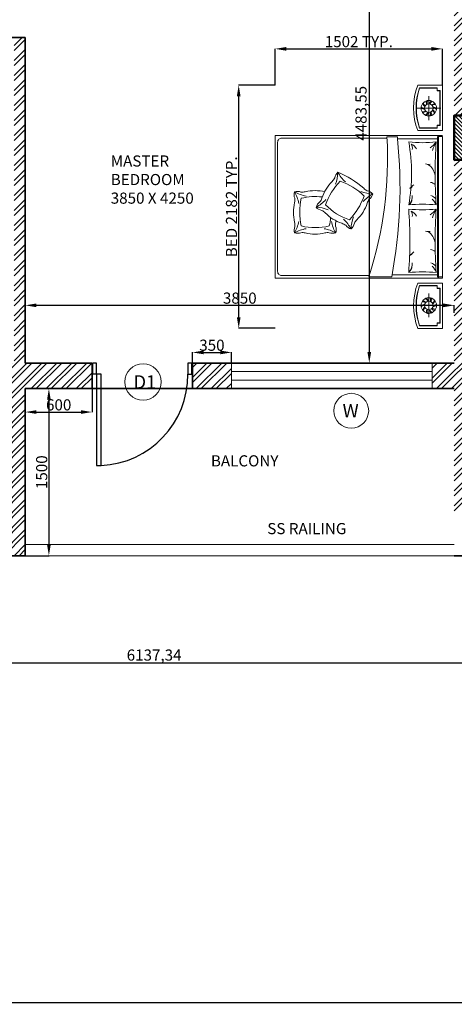
# Model space of a CAD drawing. Units: millimetres. Extents: x -3326 to 29338, y -16792 to 6002.
# Tile 5 of 21: x 7252 to 11152, y -16792 to -7951. Entities that reach past the tile are written whole.
import ezdxf

# ---------------------------------------------------------------- set-up
doc = ezdxf.new("R2010")
doc.units = ezdxf.units.MM
doc.header["$PDMODE"] = 35
doc.header["$PDSIZE"] = 5
for name, color, linetype, lineweight in [('A-ANNO-DIMS', 2, 'Continuous', 13), ('A-ANNO-SYMB', 7, 'Continuous', 18), ('A-AREA-IDEN', 7, 'Continuous', 18), ('A-COLS', 1, 'Continuous', 50), ('A-COLS-PATT', 251, 'Continuous', 13), ('A-DOOR', 3, 'Continuous', 25), ('A-FLOR-RAIL', 8, 'Continuous', 20), ('A-GLAZ', 4, 'Continuous', 18), ('A-WALL', 7, 'Continuous', 35), ('A-WALL-PATT', 252, 'Continuous', 13), ('furn', 28, 'Continuous', 18), ('txt', 7, 'Continuous', 18)]:
    doc.layers.add(name, color=color, linetype=linetype, lineweight=lineweight)
doc.styles.get("Standard").update_dxf_attribs({"font": 'arial.ttf'})
doc.dimstyles.new('ISO-25', dxfattribs={"dimtxt": 100, "dimasz": 100, "dimexe": 1.25, "dimexo": 0.625, "dimtad": 1, "dimtxsty": 'Standard', "dimcen": 2.5, "dimadec": 0, "dimazin": 0, "dimtfac": 1, "dimtmove": 0, "dimatfit": 3, "dimfxl": 1, "dimarcsym": 0})
pattern_1 = [(45, (-10476.65, 1e-12), (-67.35192, 67.35192), []), (45, (-10431.74, 1e-12), (-67.35192, 67.35192), [])]

# ---------------------------------------------------------------- blocks, each defined once
blk = doc.blocks.new('A$C0CE462CD')
for p, q in [((860, 100), (860, 0)), ((860, 0), (893.9, 0))]:
    blk.add_line(p, q)
for points in [[(860, 100), (860, 920), (818.4, 920), (818.4, 100)], [(0, 10), (6.1, 10), (6.1, 90), (0, 90)], [(893.9, 10), (900, 10), (900, 90), (893.9, 90)]]:
    blk.add_lwpolyline(points, close=True)
for points in [[(6.1, 0), (40, 0), (40, 100), (6.1, 100)], [(6.1, 100), (6.1, 0)], [(860, 100), (893.9, 100), (893.9, 0)]]:
    blk.add_lwpolyline(points)
blk.add_arc((859.1, 101.9), 819.1, 92.8508, 180.13091)
blk = doc.blocks.new('*D55')
at = {"layer": 'A-ANNO-DIMS', "color": 0, "lineweight": -2, "transparency": 16777216}
for p, q in [((7302.9, -11264), (7515.4, -11264)), ((7514.2, -11364), (7514.2, -12664)), ((7302.9, -12764), (7515.4, -12764))]:
    blk.add_line(p, q, dxfattribs=at)
at = {"layer": 'A-ANNO-DIMS', "color": 0, "transparency": 16777216}
for points in [[(7497.5, -11364), (7530.8, -11364), (7514.2, -11264)], [(7497.5, -12664), (7530.8, -12664), (7514.2, -12764)]]:
    blk.add_solid(points, dxfattribs=at)
at = {"layer": 'Defpoints', "color": 0, "transparency": 16777216}
for p in [(7302.3, -11264), (7302.3, -12764), (7514.2, -12764)]:
    blk.add_point(p, dxfattribs=at)
at = {"layer": 'A-ANNO-DIMS', "color": 0, "transparency": 16777216, "insert": (7462.5, -12014), "char_height": 100, "attachment_point": 5, "rotation": 90}
blk.add_mtext('1500', dxfattribs=at)
blk = doc.blocks.new('*D56')
at = {"layer": 'A-ANNO-DIMS', "color": 0, "lineweight": -2, "transparency": 16777216}
for p, q in [((8802.3, -11033.3), (8802.3, -10937.6)), ((8902.3, -10938.8), (9052.3, -10938.8)), ((9152.3, -11033.3), (9152.3, -10937.6))]:
    blk.add_line(p, q, dxfattribs=at)
at = {"layer": 'A-ANNO-DIMS', "color": 0, "transparency": 16777216}
for points in [[(8902.3, -10922.1), (8902.3, -10955.5), (8802.3, -10938.8)], [(9052.3, -10922.1), (9052.3, -10955.5), (9152.3, -10938.8)]]:
    blk.add_solid(points, dxfattribs=at)
at = {"layer": 'Defpoints', "color": 0, "transparency": 16777216}
for p in [(9152.3, -10938.8), (8802.3, -11034), (9152.3, -11034)]:
    blk.add_point(p, dxfattribs=at)
at = {"layer": 'A-ANNO-DIMS', "color": 0, "transparency": 16777216, "insert": (8977.3, -10887.1), "char_height": 100, "attachment_point": 5}
blk.add_mtext('350', dxfattribs=at)
blk = doc.blocks.new('*D57')
at = {"layer": 'A-ANNO-DIMS', "color": 0, "lineweight": -2, "transparency": 16777216}
for p, q in [((7302.3, -11264.6), (7302.3, -11475.4)), ((7902.3, -11264.6), (7902.3, -11475.4)), ((7402.3, -11474.2), (7802.3, -11474.2))]:
    blk.add_line(p, q, dxfattribs=at)
at = {"layer": 'A-ANNO-DIMS', "color": 0, "transparency": 16777216}
for points in [[(7402.3, -11457.5), (7402.3, -11490.8), (7302.3, -11474.2)], [(7802.3, -11457.5), (7802.3, -11490.8), (7902.3, -11474.2)]]:
    blk.add_solid(points, dxfattribs=at)
at = {"layer": 'Defpoints', "color": 0, "transparency": 16777216}
for p in [(7302.3, -11264), (7902.3, -11264), (7902.3, -11474.2)]:
    blk.add_point(p, dxfattribs=at)
at = {"layer": 'A-ANNO-DIMS', "color": 0, "transparency": 16777216, "insert": (7602.3, -11422.5), "char_height": 100, "attachment_point": 5}
blk.add_mtext('600', dxfattribs=at)
blk = doc.blocks.new('*D58')
at = {"layer": 'A-ANNO-DIMS', "color": 0, "lineweight": -2, "transparency": 16777216}
for p, q in [((7302.3, -10583), (7302.3, -10514.7)), ((7402.3, -10515.9), (11052.3, -10515.9)), ((11152.3, -10583), (11152.3, -10514.7))]:
    blk.add_line(p, q, dxfattribs=at)
at = {"layer": 'A-ANNO-DIMS', "color": 0, "transparency": 16777216}
for points in [[(7402.3, -10499.2), (7402.3, -10532.6), (7302.3, -10515.9)], [(11052.3, -10499.2), (11052.3, -10532.6), (11152.3, -10515.9)]]:
    blk.add_solid(points, dxfattribs=at)
at = {"layer": 'Defpoints', "color": 0, "transparency": 16777216}
for p in [(11152.3, -10515.9), (7302.3, -10583.6), (11152.3, -10583.6)]:
    blk.add_point(p, dxfattribs=at)
at = {"layer": 'A-ANNO-DIMS', "color": 0, "transparency": 16777216, "insert": (9227.3, -10464.2), "char_height": 100, "attachment_point": 5}
blk.add_mtext('3850', dxfattribs=at)
blk = doc.blocks.new('*D59')
at = {"layer": 'A-ANNO-DIMS', "color": 0, "lineweight": -2, "transparency": 16777216}
for p, q in [((10416, -6550.4), (10388, -6550.4)), ((10389.2, -6650.4), (10389.2, -10934)), ((10416, -11034), (10388, -11034))]:
    blk.add_line(p, q, dxfattribs=at)
at = {"layer": 'A-ANNO-DIMS', "color": 0, "transparency": 16777216}
for points in [[(10372.6, -6650.4), (10405.9, -6650.4), (10389.2, -6550.4)], [(10372.6, -10934), (10405.9, -10934), (10389.2, -11034)]]:
    blk.add_solid(points, dxfattribs=at)
at = {"layer": 'Defpoints', "color": 0, "transparency": 16777216}
for p in [(10416.6, -6550.4), (10389.2, -11034), (10416.6, -11034)]:
    blk.add_point(p, dxfattribs=at)
at = {"layer": 'A-ANNO-DIMS', "color": 0, "transparency": 16777216, "insert": (10328.5, -8792.2), "char_height": 100, "attachment_point": 5, "rotation": 90}
blk.add_mtext('4483,55', dxfattribs=at)
blk = doc.blocks.new('*D160')
at = {"layer": 'A-ANNO-DIMS', "color": 0, "lineweight": -2, "transparency": 16777216}
for p, q in [((5390, -13729), (5390, -13728.4)), ((11427.3, -13729.7), (5490, -13729.7)), ((11527.3, -13729), (11527.3, -13728.4))]:
    blk.add_line(p, q, dxfattribs=at)
at = {"layer": 'A-ANNO-DIMS', "color": 0, "transparency": 16777216}
for points in [[(5490, -13713), (5490, -13746.3), (5390, -13729.7)], [(11427.3, -13713), (11427.3, -13746.3), (11527.3, -13729.7)]]:
    blk.add_solid(points, dxfattribs=at)
at = {"layer": 'Defpoints', "color": 0, "transparency": 16777216}
for p in [(5390, -13729.7), (5390, -13729.7), (11527.3, -13729.7)]:
    blk.add_point(p, dxfattribs=at)
at = {"layer": 'A-ANNO-DIMS', "color": 0, "transparency": 16777216, "insert": (8458.6, -13668.9), "char_height": 100, "attachment_point": 5}
blk.add_mtext('6137,34', dxfattribs=at)
blk = doc.blocks.new('BED-WITH-NIGHTSTANDS')
for p, q in [((1378.9, 2083.2), (1378.9, 1869.8)), ((1272.3, 1976.5), (1485.6, 1976.5)), ((1466.8, 1702.3), (1097.4, 1702.3)), ((1455.8, 1708.6), (1455.8, 473.4)), ((1466.8, 480.5), (1049.3, 480.5)), ((1378.9, 98.8), (1378.9, 312.2)), ((1272.2, 205.5), (1485.6, 205.5))]:
    blk.add_line(p, q)
for points in [[(1279.5, 2182), (1501.4, 2182), (1501.4, 1775.2), (1279.5, 1775.2, -0.181818)], [(1097.4, 1719.6), (1097.4, 1702.3, -0.072944), (1045.8, 463.1), (840.6, 463.1, 0.092568), (1003.3, 1719.6)], [(1198.4, 1674.1, 0.058596), (1445.6, 1674.1, 0.036889), (1445.6, 1107.7, 0.052163), (1198.4, 1107.7, 0.093111)], [(1198.4, 1070.9, 0.058596), (1445.6, 1070.9, 0.036648), (1445.6, 500.8, 0.052163), (1198.4, 500.8, 0.036967)], [(1279.6, 0), (1501.5, 0), (1501.5, 406.8), (1279.6, 406.8, 0.181818)]]:
    blk.add_lwpolyline(points, format="xyb", close=True)
for points in [[(1454.8, 1797.4), (1295, 1797.4, -0.167087), (1295, 2159.8), (1454.8, 2159.8)], [(1454.8, 1799.6), (1296.6, 1799.6, -0.165559), (1296.6, 2157.6), (1454.8, 2157.6)], [(1003.9, 1708.6), (59.2, 1708.6, 0.414214), (22.2, 1671.6), (22.2, 510.4, 0.414214), (59.2, 473.4), (844.2, 473.4)], [(540, 1293.1, 0.091296), (562.8, 1401.4, 0.091296), (630.7, 1314.1, 0.091296)], [(583.2, 1320, 0.111006), (451.8, 1108.7, 0.119549), (665.6, 975.5, 0.107813), (797.5, 1186.1)], [(797.2, 1187.3, 0.121865), (583.2, 1319.9, 0.121865)], [(211.2, 1122.2, 0.091296), (173.3, 1226.2, 0.091296), (277.2, 1187.9, 0.091296)], [(233.7, 1167.8, 0.111006), (234, 919, 0.119549), (485.8, 919, 0.033212), (497.4, 995.5)], [(475.6, 1065.1, 0.091296), (367.2, 1087.5, 0.091296), (454.4, 1155.8)], [(768.3, 1228.3, 0.091296), (876.7, 1205.8, 0.091296), (789.5, 1137.6, 0.091296)], [(367.2, 1087.5, 0.159461), (418, 1058.9, -0.076283), (449.6, 1036.2, 0.115075), (598.7, 943.3, -0.076283), (633, 924.9, 0.159461), (681.1, 892)], [(703.9, 1000.2, 0.091296), (681.1, 892, 0.091296), (613.2, 979.3, 0.091296)], [(277.2, 894.6, 0.091296), (173.3, 856.3, 0.091296), (211.2, 960.3)], [(505.3, 960.3, 0.091296), (543.2, 856.3, 0.091296), (439.3, 894.6, 0.091296)], [(173.3, 856.3, 0.159461), (231.6, 858.9, -0.076283), (270.5, 856.3, 0.115075), (446, 856.3, -0.076283), (484.9, 858.9, 0.159461), (543.2, 856.3)], [(1454.9, 384.6), (1295.1, 384.6, 0.167087), (1295.1, 22.2), (1454.9, 22.2)], [(1454.9, 382.4), (1296.7, 382.4, 0.165559), (1296.7, 24.4), (1454.9, 24.4)]]:
    blk.add_lwpolyline(points, format="xyb")
for points in [[(1479.2, 2133.2), (1452.6, 2133.2), (1452.6, 2159.8)], [(1479.2, 2135.4), (1454.8, 2135.4), (1454.8, 2159.8)], [(1477, 2135.4), (1477, 1821.8)], [(1479.2, 2135.4), (1479.2, 1821.8)], [(1479.2, 1824), (1452.6, 1824), (1452.6, 1797.4)], [(1479.2, 1821.8), (1454.8, 1821.8), (1454.8, 1797.4)], [(1501.5, 1730.8), (0, 1730.8), (0, 451.2), (1501.5, 451.2)], [(1501.5, 463.1), (1466.8, 463.1), (1466.8, 1723.4), (1501.5, 1723.4), (1501.5, 451.2)], [(1479.3, 358), (1452.7, 358), (1452.7, 384.6)], [(1479.3, 360.2), (1454.9, 360.2), (1454.9, 384.6)], [(1477.1, 46.6), (1477.1, 360.2)], [(1479.3, 46.6), (1479.3, 360.2)], [(1479.3, 48.8), (1452.7, 48.8), (1452.7, 22.2)], [(1479.3, 46.6), (1454.9, 46.6), (1454.9, 22.2)]]:
    blk.add_lwpolyline(points)
for centre, radius in [((1378.9, 1976.5), 69.7), ((1378.9, 1976.5), 37.8), ((1378.9, 205.5), 69.7), ((1378.9, 205.5), 37.8)]:
    blk.add_circle(centre, radius)
for centre, radius, start, end in [((1400.9, 2024.2), 44.8, 154.17003, 200.48975), ((1396.5, 2024.6), 34.1, 142.30017, 202.53802), ((1424.8, 2002.2), 44.8, 118.17003, 164.48975), ((1421.4, 2005.1), 34.1, 106.30017, 166.53802), ((1340.3, 2012.2), 44.8, 226.17003, 272.48975), ((1338.5, 2008.1), 34.1, 214.30017, 274.53802), ((1327.7, 1978.3), 34.1, 250.30017, 310.53802), ((1326.7, 1982.7), 44.8, 262.17003, 308.48975), ((1368.7, 2028), 44.8, 190.17003, 236.48975), ((1364.8, 2025.8), 34.1, 178.30017, 238.53802), ((1431.1, 1970.3), 44.8, 82.17003, 128.48975), ((1430.1, 1974.7), 34.1, 70.30017, 130.53802), ((1393, 1927.2), 34.1, 358.30017, 58.53802), ((1389.2, 1925), 44.8, 10.17003, 56.48975), ((1417.5, 1940.8), 44.8, 46.17003, 92.48975), ((1419.3, 1944.9), 34.1, 34.30017, 94.53802), ((1336.4, 1947.9), 34.1, 286.30017, 346.53802), ((1333.1, 1950.8), 44.8, 298.17003, 344.48975), ((1361.4, 1928.3), 34.1, 322.30017, 22.53802), ((1356.9, 1928.8), 44.8, 334.17003, 20.48975), ((1478, 1708.6), 22.2, 90, 180), ((1175.6, 1619.4), 56.2, 346.48229, 38.55627), ((1192.7, 1576.7), 82.2, 24.2916, 70.9896), ((1214.5, 1859.4), 296.3, 306.49353, 321.27919), ((1652.3, 1542.6), 244.9, 147.53791, 167.5233), ((1375.3, 1532.7), 61.4, 245.89274, 286.11919), ((1299.1, 1354.7), 137.1, 6.68493, 58.3182), ((419.7, 1408.4), 128.4, 315.77185, 333.2208), ((626.3, 1332.5), 93.8, 132.65224, 168.89294), ((256.3, 651.7), 810, 48.38179, 67.76439), ((785.6, 1046.2), 386.5, 135.13065, 161.38844), ((884.1, 1348.9), 128.4, 225.58539, 243.03435), ((1208.9, 1279), 20.7, 263.75428, 347.21866), ((1026.5, 1507.4), 308.8, 306.20852, 315.08491), ((1377, 1216.1), 96.2, 51.81741, 79.89867), ((263.7, 1201.2), 93.8, 164.57915, 200.81985), ((198.5, 1135.9), 93.8, 69.36661, 105.60731), ((48.2, 1156.4), 128.4, 347.69876, 5.14771), ((242.7, 1351.6), 128.4, 265.03874, 282.4877), ((360.8, 659.2), 524.3, 83.19556, 104.02838), ((358.2, 849.8), 386.5, 76.87111, 103.12889), ((298.1, 1211.9), 128.4, 323.29829, 340.74724), ((807.5, 1142.5), 93.8, 42.46578, 78.70648), ((947.4, 1081.9), 128.4, 143.29829, 160.74724), ((789.7, 1230.6), 90.5, 307.29372, 344.09733), ((1127.7, 1179.9), 101.1, 314.40604, 6.83423), ((1163, 1161), 64, 303.63488, 0.84559), ((1363.4, 1094.5), 103.5, 40.53543, 70.35581), ((1276.2, 1030), 186.4, 24.64565, 44.15848), ((550.3, 1042.5), 386.5, 167.05756, 193.31535), ((468.2, 1051.5), 107.3, 128.77541, 160.35713), ((460, 1247.6), 386.5, 315.13065, 341.38844), ((1214.5, 1256.2), 296.3, 306.49353, 321.27919), ((1652.3, 939.4), 244.9, 147.53791, 167.5233), ((825.9, 885.4), 128.4, 135.77185, 153.2208), ((1175.6, 1016.2), 56.2, 346.48229, 38.55627), ((1192.7, 973.5), 82.2, 24.2916, 70.9896), ((278.1, 879.2), 107.3, 160.70232, 192.28404), ((48.9, 925.3), 128.4, 355.2252, 12.67415), ((669.5, 927.3), 128.4, 167.69876, 185.14771), ((461.1, 884), 86.6, 341.39955, 21.57741), ((167.4, 1041.2), 386.5, 347.05756, 348.7033), ((626.1, 958.8), 86.6, 309.47264, 349.6505), ((1375.3, 929.5), 61.4, 245.89274, 286.11919), ((1299.1, 751.6), 137.1, 6.68493, 58.3182), ((1377, 612.9), 96.2, 51.81741, 79.89867), ((1208.9, 675.8), 20.7, 263.75428, 347.21866), ((1026.5, 904.2), 308.8, 306.20852, 315.08491), ((1127.7, 576.7), 101.1, 314.40604, 6.83423), ((1163, 557.8), 64, 303.63488, 0.84559), ((1363.4, 491.3), 103.5, 40.53543, 70.35581), ((1276.2, 426.8), 186.4, 24.64565, 44.15848), ((1478, 473.4), 22.2, 180, 270), ((1336.4, 234.2), 34.1, 13.46198, 73.69983), ((1333, 231.2), 44.8, 15.51025, 61.82997), ((1361.4, 253.7), 34.1, 337.46198, 37.69983), ((1356.9, 253.2), 44.8, 339.51025, 25.82997), ((1340.3, 169.8), 44.8, 87.51025, 133.82997), ((1338.5, 173.9), 34.1, 85.46198, 145.69983), ((1327.7, 203.7), 34.1, 49.46198, 109.69983), ((1326.7, 199.3), 44.8, 51.51025, 97.82997), ((1368.6, 154), 44.8, 123.51025, 169.82997), ((1364.8, 156.2), 34.1, 121.46198, 181.69983), ((1430.1, 207.3), 34.1, 229.46198, 289.69983), ((1393, 254.8), 34.1, 301.46198, 1.69983), ((1389.2, 257.1), 44.8, 303.51025, 349.82997), ((1417.5, 241.2), 44.8, 267.51025, 313.82997), ((1419.3, 237.1), 34.1, 265.46198, 325.69983), ((1402.8, 152.7), 44.8, 159.51025, 205.82997), ((1398.4, 152.3), 34.1, 157.46198, 217.69983), ((1426.7, 174.7), 44.8, 195.51025, 241.82997), ((1423.3, 171.8), 34.1, 193.46198, 253.69983), ((1433, 206.6), 44.8, 231.51025, 277.82997)]:
    blk.add_arc(centre, radius, start, end)
blk = doc.blocks.new('TAG-D1')
blk.add_circle((163.3, 163.3), 163.3)
at = {"insert": (78, 223.5), "char_height": 120, "attachment_point": 1}
blk.add_mtext_dynamic_manual_height_columns('D1', width=137.943, gutter_width=12.5, heights=[0], dxfattribs=at)
blk = doc.blocks.new('TAG-W')
blk.add_circle((156.8, 156.8), 156.8)
at = {"insert": (79.7, 216.8), "char_height": 120, "attachment_point": 1}
blk.add_mtext_dynamic_manual_height_columns('W', width=376.575, gutter_width=12.5, heights=[0], dxfattribs=at)
blk = doc.blocks.new('GLAZ-1800x80')
for p, q in [((0, 80), (1800, 80)), ((0, 0), (1800, 0))]:
    blk.add_line(p, q)
blk = doc.blocks.new('*D213')
at = {"layer": 'A-ANNO-DIMS', "color": 0, "lineweight": -2, "transparency": 16777216}
for p, q in [((9544.2, -8540.5), (9216.3, -8540.5)), ((9217.5, -10622.5), (9217.5, -8640.5)), ((9544.2, -10722.5), (9216.3, -10722.5))]:
    blk.add_line(p, q, dxfattribs=at)
at = {"layer": 'A-ANNO-DIMS', "color": 0, "transparency": 16777216}
for points in [[(9200.9, -8640.5), (9234.2, -8640.5), (9217.5, -8540.5)], [(9200.9, -10622.5), (9234.2, -10622.5), (9217.5, -10722.5)]]:
    blk.add_solid(points, dxfattribs=at)
at = {"layer": 'Defpoints', "color": 0, "transparency": 16777216}
for p in [(9217.5, -8540.5), (9544.8, -8540.5), (9544.8, -10722.5)]:
    blk.add_point(p, dxfattribs=at)
at = {"layer": 'A-ANNO-DIMS', "color": 0, "transparency": 16777216, "insert": (9165.8, -9631.5), "char_height": 100, "attachment_point": 5, "rotation": 90}
blk.add_mtext('BED 2182 TYP.', dxfattribs=at)
blk = doc.blocks.new('*D214')
at = {"layer": 'A-ANNO-DIMS', "color": 0, "lineweight": -2, "transparency": 16777216}
for p, q in [((9544.8, -8539.9), (9544.8, -8212)), ((9644.8, -8213.2), (10946.3, -8213.2)), ((11046.3, -8539.9), (11046.3, -8212))]:
    blk.add_line(p, q, dxfattribs=at)
at = {"layer": 'A-ANNO-DIMS', "color": 0, "transparency": 16777216}
for points in [[(9644.8, -8196.5), (9644.8, -8229.9), (9544.8, -8213.2)], [(10946.3, -8196.5), (10946.3, -8229.9), (11046.3, -8213.2)]]:
    blk.add_solid(points, dxfattribs=at)
at = {"layer": 'Defpoints', "color": 0, "transparency": 16777216}
for p in [(11046.3, -8213.2), (9544.8, -8540.5), (11046.3, -8540.5)]:
    blk.add_point(p, dxfattribs=at)
at = {"layer": 'A-ANNO-DIMS', "color": 0, "transparency": 16777216, "insert": (10295.6, -8161.5), "char_height": 100, "attachment_point": 5}
blk.add_mtext('1502 TYP.', dxfattribs=at)
blk = doc.blocks.new('*D235')
at = {"layer": 'A-ANNO-DIMS', "color": 0, "lineweight": -2, "transparency": 16777216}
for p, q in [((-617.7, -12764.6), (-617.7, -16776.1)), ((29282.3, -12764.6), (29282.3, -16776.1)), ((-517.7, -16774.9), (29182.3, -16774.9))]:
    blk.add_line(p, q, dxfattribs=at)
at = {"layer": 'A-ANNO-DIMS', "color": 0, "transparency": 16777216}
for points in [[(-517.7, -16758.2), (-517.7, -16791.6), (-617.7, -16774.9)], [(29182.3, -16758.2), (29182.3, -16791.6), (29282.3, -16774.9)]]:
    blk.add_solid(points, dxfattribs=at)
at = {"layer": 'Defpoints', "color": 0, "transparency": 16777216}
for p in [(-617.7, -12764), (29282.3, -12764), (29282.3, -16774.9)]:
    blk.add_point(p, dxfattribs=at)
at = {"layer": 'A-ANNO-DIMS', "color": 0, "transparency": 16777216, "insert": (14332.3, -16723.2), "char_height": 100, "attachment_point": 5}
blk.add_mtext('29900', dxfattribs=at)

msp = doc.modelspace()

# ---------------------------------------------------------------- hatches: boundary and pattern name
at = {"layer": 'A-COLS-PATT'}
h = msp.add_hatch(dxfattribs=at)
h.set_pattern_fill('ANSI31', color=256, scale=8, angle=-90)
h.set_pattern_definition([(315, (18358.179, 32910.899), (17.960512, 17.960512), [])])
h.paths.add_polyline_path([(11151.174, -8810.401), (11151.174, -9210.401), (11751.174, -9210.401), (11751.174, -8810.401)])
at = {"layer": 'A-WALL-PATT'}
h = msp.add_hatch(dxfattribs=at)
h.set_pattern_fill('ANSI32', color=256, scale=10)
h.set_pattern_definition(pattern_1)
h.paths.add_polyline_path([(12212.301, -1983.952), (11640.861, -1983.952), (11640.861, -2213.952), (12212.301, -2213.952)])
h.paths.add_polyline_path([(14712.301, -1983.952), (14012.301, -1983.952), (14012.301, -2213.952), (14712.301, -2213.952)])
h.paths.add_polyline_path([(17012.301, -1983.952), (16512.301, -1983.952), (16512.301, -2213.952), (17012.301, -2213.952)])
h.paths.add_polyline_path([(11382.301, -2383.952), (11040.861, -2383.952), (7302.301, -2383.952), (7302.301, -1935.766), (7217.026, -1935.766), (7202.301, -1933.952), (7202.301, -2483.952), (7302.301, -2483.952), (11152.301, -2483.952), (11152.301, -2833.952), (11283.549, -2833.952), (11283.549, -2830.395), (11363.875, -2830.395), (11382.301, -2833.952)])
h.paths.add_polyline_path([(11382.301, -3733.952), (11363.875, -3733.952), (11363.875, -3734.058), (11283.549, -3734.058), (11152.301, -3733.952), (11152.301, -6450.401), (11382.301, -6450.401)])
h.paths.add_polyline_path([(13462.301, -6450.401), (12606.738, -6450.401), (11382.301, -6450.401), (11382.301, -6680.401), (12606.738, -6680.401), (13462.301, -6680.401)])
h.paths.add_polyline_path([(11382.301, -7050.401), (11152.301, -7050.401), (11152.301, -8810.401), (11382.301, -8810.401)])
h.paths.add_polyline_path([(13462.301, -8980.401), (11751.174, -8980.401), (11751.174, -9210.401), (13462.301, -9210.401)])
h.paths.add_polyline_path([(13962.301, -6850.401), (13732.301, -6850.401), (13732.301, -7350.401), (13962.301, -7350.401)])
h.paths.add_polyline_path([(13962.301, -8309.482), (13732.301, -8309.482), (13732.301, -8809.482), (13962.301, -8809.482)])
h.paths.add_polyline_path([(15712.301, -12533.952), (12902.301, -12533.952), (12902.301, -12763.952), (15712.301, -12763.952)])
h.paths.add_polyline_path([(11508.301, -9211.585), (11382.301, -9211.585), (11152.301, -9211.585), (11152.301, -11033.952), (10952.301, -11033.952), (10952.301, -11263.952), (11152.301, -11263.952), (11152.301, -12361.585), (11508.301, -12361.585)])
h.paths.add_polyline_path([(12002.301, -12533.952), (11902.301, -12533.952), (11902.301, -12761.585), (11152.301, -12761.585), (11152.301, -12763.952), (11902.301, -12763.952), (12002.301, -12763.952)])
h.paths.add_polyline_path([(17112.301, -12533.952), (16912.301, -12533.952), (16912.301, -12763.952), (17112.301, -12763.952)])
h.paths.add_polyline_path([(11382.301, 3596.048), (11152.301, 3596.048), (11152.301, 2096.048), (11382.301, 2096.048)])
h.paths.add_polyline_path([(11382.301, 1496.048), (11152.301, 1496.048), (11152.301, -1983.952), (11382.301, -1983.952)])
h = msp.add_hatch(dxfattribs=at)
h.set_pattern_fill('ANSI32', color=256, scale=10)
h.set_pattern_definition(pattern_1)
h.paths.add_polyline_path([(7302.301, -11263.952), (7902.301, -11263.952), (7902.301, -11033.952), (7302.301, -11033.952), (7302.301, -8110.991), (7202.301, -8110.991), (7202.301, -11033.952), (6672.301, -11033.952), (6672.301, -11263.952), (7072.301, -11263.952), (7072.301, -12763.952), (7302.301, -12763.952)])
h.paths.add_polyline_path([(9152.301, -11033.952), (8802.301, -11033.952), (8802.301, -11044.19), (8802.545, -11044.19), (8802.545, -11124.19), (8802.301, -11263.952), (9152.301, -11263.952)])
h.paths.add_polyline_path([(3712.301, -8110.991), (3612.301, -8110.991), (3612.301, -11033.952), (3282.301, -11033.952), (3282.301, -11263.952), (3612.301, -11263.952), (3612.301, -12763.952), (3842.301, -12763.952), (3842.301, -11263.952), (4092.301, -11263.952), (4092.301, -11033.952), (3842.301, -11033.952), (3712.301, -11033.952)])
h.paths.add_polyline_path([(5172.301, -11033.952), (4692.301, -11033.952), (4692.301, -11263.952), (5172.301, -11263.952)])
h.paths.add_polyline_path([(6072.301, -11033.952), (5572.301, -11033.952), (5572.301, -11263.952), (6072.301, -11263.952)])
h.paths.add_polyline_path([(6072.301, -11263.952), (5972.301, -11263.952), (5972.301, -11663.952), (6072.301, -11663.952)])
h.paths.add_polyline_path([(4792.301, -11263.952), (4692.301, -11263.952), (4692.301, -11663.952), (4792.301, -11663.952)])
h.paths.add_polyline_path([(6402.301, -8110.991), (6272.301, -8110.991), (5572.301, -8110.991), (5572.301, -7200.401), (5342.301, -7200.401), (5342.301, -8110.991), (4642.301, -8110.991), (4512.301, -8110.991), (4512.301, -8210.991), (4642.301, -8210.991), (5342.301, -8210.991), (5342.301, -10513.952), (5572.301, -10513.952), (5572.301, -8210.991), (6272.301, -8210.991), (6402.301, -8210.991)])
h.paths.add_polyline_path([(232.301, -11033.952), (-217.699, -11033.952), (-217.699, -11263.952), (232.301, -11263.952)])
h.paths.add_polyline_path([(1482.301, -11033.952), (1132.301, -11033.952), (1132.301, -11044.8), (1132.987, -11044.8), (1132.987, -11124.8), (1132.301, -11263.952), (1482.301, -11263.952)])
h.paths.add_polyline_path([(-387.699, -11263.952), (-617.699, -11263.952), (-617.699, -12763.952), (-438.882, -12763.952), (-387.699, -12763.952)])
h.paths.add_polyline_path([(-387.699, -7150.401), (-215.519, -7150.401), (-215.519, -7050.401), (-617.699, -7050.401), (-617.699, -10763.952), (-387.699, -10763.952)])
h.paths.add_polyline_path([(1512.301, -5983.952), (1282.301, -5983.952), (1282.301, -6450.401), (-215.519, -6450.401), (-215.519, -6550.401), (4073.51, -6550.401), (4073.51, -6450.401), (1512.301, -6450.401)])
h.paths.add_polyline_path([(5773.51, -6450.401), (5573.51, -6450.401), (5573.51, -6550.401), (5773.51, -6550.401)])
h.paths.add_polyline_path([(5173.51, -6450.401), (4973.51, -6450.401), (4973.51, -6550.401), (5173.51, -6550.401)])
h.paths.add_polyline_path([(10982.301, -6450.401), (6673.51, -6450.401), (6673.51, -6550.401), (10982.301, -6550.401)])

# ---------------------------------------------------------------- linework, layer by layer
at = {"layer": 'A-COLS'}
msp.add_lwpolyline([(11751.174, -8810.401), (11751.174, -9210.401), (11151.174, -9210.401), (11151.174, -8810.401)], close=True, dxfattribs=at)
at = {"layer": 'A-FLOR-RAIL'}
for p, q in [((11152.301, -12663.952), (7302.301, -12663.952)), ((11152.301, -12763.952), (7302.301, -12763.952))]:
    msp.add_line(p, q, dxfattribs=at)
at = {"layer": 'A-GLAZ'}
for p, q in [((9152.301, -11263.952), (9152.301, -11033.952)), ((10952.301, -11263.952), (10952.301, -11033.952))]:
    msp.add_line(p, q, dxfattribs=at)
at = {"layer": 'A-WALL'}
for p, q in [((7302.301, -8110.991), (7072.301, -8110.991)), ((7302.301, -8110.991), (7302.301, -11033.952)), ((7902.301, -11033.952), (7302.301, -11033.952)), ((7902.301, -11263.952), (7902.301, -11033.952)), ((11152.301, -11033.952), (8802.301, -11033.952)), ((8802.301, -11263.952), (8802.301, -11033.952)), ((11152.301, -11263.952), (7302.301, -11263.952)), ((7302.301, -11263.952), (7302.301, -12763.952)), ((7302.301, -12763.952), (7072.301, -12763.952)), ((11902.301, -12763.952), (11152.301, -12763.952))]:
    msp.add_line(p, q, dxfattribs=at)

# ---------------------------------------------------------------- block references
at = {"layer": 'A-ANNO-SYMB'}
for name, p in [('TAG-D1', (8196.028, -11366.978)), ('TAG-W', (10070.417, -11619.541))]:
    msp.add_blockref(name, p, dxfattribs=at)
at = {"layer": 'A-DOOR', "rotation": 180}
msp.add_blockref('A$C0CE462CD', (8802.545, -11034.19), dxfattribs=at)
at = {"layer": 'A-GLAZ'}
msp.add_blockref('GLAZ-1800x80', (9152.301, -11188.952), dxfattribs=at)
at = {"layer": 'furn'}
msp.add_blockref('BED-WITH-NIGHTSTANDS', (9544.822, -10722.508), dxfattribs=at)

# ---------------------------------------------------------------- texts
at = {"layer": 'A-AREA-IDEN', "char_height": 100, "attachment_point": 1}
for s, insert in [('MASTER\\PBEDROOM\\P3850 X 4250', (8069.267, -9170.112)), ('BALCONY', (8968.169, -11862.223))]:
    msp.add_mtext_dynamic_manual_height_columns(s, width=1168.90663, gutter_width=12.5, heights=[0], dxfattribs=dict(at, insert=insert))
at = {"layer": 'txt', "insert": (9474.078, -12470.525), "char_height": 100, "attachment_point": 1}
msp.add_mtext_dynamic_manual_height_columns('SS RAILING', width=1168.90663, gutter_width=12.5, heights=[0], dxfattribs=at)

# ---------------------------------------------------------------- dimensions: what is measured, and where the dimension line sits
at = {"layer": 'A-ANNO-DIMS'}
for base, p1, p2, picture, middle in [((10389.237, -11033.952), (10416.582, -6550.401), (10416.582, -11033.952), '*D59', (10328.517, -8792.177)), ((7514.162, -12763.952), (7302.301, -11263.952), (7302.301, -12763.952), '*D55', (7462.48, -12013.952))]:
    dim = msp.add_linear_dim(base=base, p1=p1, p2=p2, angle=90, dimstyle='ISO-25', override={"dimclrd": 0, "dimclre": 0, "dimclrt": 0}, dxfattribs=at)
    dim.commit()
    dim.dimension.update_dxf_attribs({"geometry": picture, "text_midpoint": middle})
dim = msp.add_linear_dim(base=(11046.337, -8213.203), p1=(9544.822, -8540.503), p2=(11046.337, -8540.503), text='<> TYP.', dimstyle='ISO-25', override={"dimdec": 0, "dimlfac": 1, "dimrnd": 0, "dimzin": 0, "dimdsep": 46, "dimlunit": 2}, dxfattribs=at)
dim.commit()
dim.dimension.update_dxf_attribs({"geometry": '*D214', "text_midpoint": (10295.58, -8161.521)})
dim = msp.add_linear_dim(base=(9217.522, -8540.503), p1=(9544.822, -10722.507), p2=(9544.822, -8540.503), angle=90, text='BED <> TYP.', dimstyle='ISO-25', override={"dimdec": 0, "dimlfac": 1, "dimrnd": 0, "dimzin": 0, "dimdsep": 46, "dimlunit": 2}, dxfattribs=at)
dim.commit()
dim.dimension.update_dxf_attribs({"geometry": '*D213', "text_midpoint": (9165.839, -9631.505)})
for base, p1, p2, override, picture, middle in [((11152.301, -10515.904), (7302.301, -10583.602), (11152.301, -10583.602), {"dimclrd": 0, "dimclre": 0, "dimclrt": 0}, '*D58', (9227.301, -10464.188)), ((9152.301, -10938.801), (8802.301, -11033.952), (9152.301, -11033.952), {"dimclrd": 0, "dimclre": 0, "dimclrt": 0}, '*D56', (8977.301, -10887.084)), ((7902.301, -11474.16), (7302.301, -11263.952), (7902.301, -11263.952), {"dimclrd": 0, "dimclre": 0, "dimclrt": 0}, '*D57', (7602.301, -11422.478)), ((29282.301, -16774.892), (-617.699, -12763.952), (29282.301, -12763.952), {"dimdec": 0, "dimlfac": 1, "dimrnd": 0, "dimzin": 0, "dimdsep": 46, "dimlunit": 2}, '*D235', (14332.301, -16723.21)), ((5389.9656, -13729.6686), (11527.3007, -13729.6686), (5389.9656, -13729.6686), {"dimclrd": 0, "dimclre": 0, "dimclrt": 0}, '*D160', (8458.6331, -13668.9481))]:
    dim = msp.add_linear_dim(base=base, p1=p1, p2=p2, dimstyle='ISO-25', override=override, dxfattribs=at)
    dim.commit()
    dim.dimension.update_dxf_attribs({"geometry": picture, "text_midpoint": middle})

doc.saveas('drawing.dxf')
